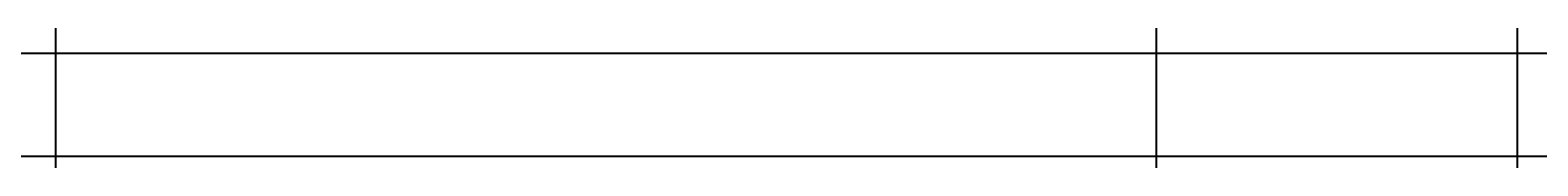
# Model space of a CAD drawing. Units: inches. Extents: x 35362 to 73946, y 43607 to 67532.
# Tile 79 of 134: x 50119 to 51337, y 47206 to 47304. Entities that reach past the tile are written whole.
import ezdxf

# ---------------------------------------------------------------- set-up
doc = ezdxf.new("R2010")
doc.units = ezdxf.units.IN
doc.header["$MEASUREMENT"] = 0
doc.layers.add('A-ANNO-DIMS', color=2, linetype='Continuous', lineweight=18)
doc.styles.get("Standard").update_dxf_attribs({"font": 'arial.ttf'})
doc.dimstyles.get("Standard").update_dxf_attribs({"dimtxt": 0.18, "dimasz": 0.18, "dimexe": 0.18, "dimexo": 0.0625, "dimgap": 0.09, "dimtad": 0, "dimtih": 1, "dimtoh": 1, "dimdec": 4, "dimzin": 0, "dimdsep": 46, "dimtxsty": 'Standard', "dimcen": 0.09, "dimadec": 0, "dimazin": 0, "dimtfac": 1, "dimtdec": 4, "dimtofl": 0, "dimtmove": 0, "dimatfit": 3, "dimfxl": 1, "dimtolj": 1, "dimtzin": 0, "dimarcsym": 0})

# ---------------------------------------------------------------- blocks, each defined once
blk = doc.blocks.new('*D11')
at = {"layer": 'A-ANNO-DIMS', "color": 0, "lineweight": -2, "transparency": 16777216}
for p, q in [((47978.7, 56028.8), (47978.7, 43606.7)), ((53109.8, 56028.8), (53109.8, 43606.7)), ((47978.8, 43606.9), (50543.9, 43606.9)), ((53109.6, 43606.9), (50544.6, 43606.9))]:
    blk.add_line(p, q, dxfattribs=at)
at = {"layer": 'A-ANNO-DIMS', "color": 0, "transparency": 16777216}
for points in [[(47978.8, 43606.9), (47978.8, 43606.8), (47978.7, 43606.9)], [(53109.6, 43606.9), (53109.6, 43606.8), (53109.8, 43606.9)]]:
    blk.add_solid(points, dxfattribs=at)
at = {"layer": 'Defpoints', "color": 0, "transparency": 16777216}
for p in [(47978.7, 56028.8), (53109.8, 56028.8), (53109.8, 43606.9)]:
    blk.add_point(p, dxfattribs=at)
at = {"layer": 'A-ANNO-DIMS', "color": 0, "transparency": 16777216, "insert": (50544.2, 43606.9), "char_height": 0.18, "attachment_point": 5}
blk.add_mtext('\\A1;5131', dxfattribs=at)
blk = doc.blocks.new('*D13')
at = {"layer": 'A-ANNO-DIMS', "color": 0, "lineweight": -2, "transparency": 16777216}
for p, q in [((48373.5, 51694), (48373.5, 43606.7)), ((51029, 51694), (51029, 43606.7)), ((48373.7, 43606.9), (49700.8, 43606.9)), ((51028.9, 43606.9), (49701.7, 43606.9))]:
    blk.add_line(p, q, dxfattribs=at)
at = {"layer": 'A-ANNO-DIMS', "color": 0, "transparency": 16777216}
for points in [[(48373.7, 43606.9), (48373.7, 43606.8), (48373.5, 43606.9)], [(51028.9, 43606.9), (51028.9, 43606.8), (51029, 43606.9)]]:
    blk.add_solid(points, dxfattribs=at)
at = {"layer": 'Defpoints', "color": 0, "transparency": 16777216}
for p in [(48373.5, 51694.1), (51029, 51694.1), (51029, 43606.9)]:
    blk.add_point(p, dxfattribs=at)
at = {"layer": 'A-ANNO-DIMS', "color": 0, "transparency": 16777216, "insert": (49701.3, 43606.9), "char_height": 0.18, "attachment_point": 5}
blk.add_mtext('\\A1;2655.6', dxfattribs=at)
blk = doc.blocks.new('*D17')
at = {"layer": 'A-ANNO-DIMS', "color": 0, "lineweight": -2, "transparency": 16777216}
for p, q in [((49923.3, 61293.2), (49923.3, 43606.7)), ((51913.9, 61293.2), (51913.9, 43606.7)), ((49923.5, 43606.9), (50918.2, 43606.9)), ((51913.8, 43606.9), (50919.1, 43606.9))]:
    blk.add_line(p, q, dxfattribs=at)
at = {"layer": 'A-ANNO-DIMS', "color": 0, "transparency": 16777216}
for points in [[(49923.5, 43606.9), (49923.5, 43606.8), (49923.3, 43606.9)], [(51913.8, 43606.9), (51913.8, 43606.8), (51913.9, 43606.9)]]:
    blk.add_solid(points, dxfattribs=at)
at = {"layer": 'Defpoints', "color": 0, "transparency": 16777216}
for p in [(49923.3, 61293.3), (51913.9, 61293.3), (51913.9, 43606.9)]:
    blk.add_point(p, dxfattribs=at)
at = {"layer": 'A-ANNO-DIMS', "color": 0, "transparency": 16777216, "insert": (50918.6, 43606.9), "char_height": 0.18, "attachment_point": 5}
blk.add_mtext('\\A1;1990.6', dxfattribs=at)
blk = doc.blocks.new('*D43')
at = {"layer": 'A-ANNO-DIMS', "color": 0, "lineweight": -2, "transparency": 16777216}
for p, q in [((62004.7, 47625.2), (35361.8, 47625.2)), ((35361.9, 47625), (35361.9, 47416.9)), ((35361.9, 47208.4), (35361.9, 47416.5)), ((62004.7, 47208.2), (35361.8, 47208.2))]:
    blk.add_line(p, q, dxfattribs=at)
at = {"layer": 'A-ANNO-DIMS', "color": 0, "transparency": 16777216}
for points in [[(35361.9, 47625), (35362, 47625), (35361.9, 47625.2)], [(35361.9, 47208.4), (35362, 47208.4), (35361.9, 47208.2)]]:
    blk.add_solid(points, dxfattribs=at)
at = {"layer": 'Defpoints', "color": 0, "transparency": 16777216}
for p in [(62004.7, 47625.2), (35361.9, 47208.2), (62004.7, 47208.2)]:
    blk.add_point(p, dxfattribs=at)
at = {"layer": 'A-ANNO-DIMS', "color": 0, "transparency": 16777216, "insert": (35361.9, 47416.7), "char_height": 0.18, "attachment_point": 5}
blk.add_mtext('\\A1;416.9', dxfattribs=at)
blk = doc.blocks.new('*D67')
at = {"layer": 'A-ANNO-DIMS', "color": 0, "lineweight": -2, "transparency": 16777216}
for p, q in [((56873.5, 53351.5), (35361.8, 53351.5)), ((35361.9, 53351.3), (35361.9, 49400.9)), ((35361.9, 45450.1), (35361.9, 49400.5)), ((53793.6, 45449.9), (35361.8, 45449.9))]:
    blk.add_line(p, q, dxfattribs=at)
at = {"layer": 'A-ANNO-DIMS', "color": 0, "transparency": 16777216}
for points in [[(35361.9, 53351.3), (35362, 53351.3), (35361.9, 53351.5)], [(35361.9, 45450.1), (35362, 45450.1), (35361.9, 45449.9)]]:
    blk.add_solid(points, dxfattribs=at)
at = {"layer": 'Defpoints', "color": 0, "transparency": 16777216}
for p in [(35361.9, 53351.5), (56873.6, 53351.5), (53793.6, 45449.9)]:
    blk.add_point(p, dxfattribs=at)
at = {"layer": 'A-ANNO-DIMS', "color": 0, "transparency": 16777216, "insert": (35361.9, 49400.7), "char_height": 0.18, "attachment_point": 5}
blk.add_mtext('\\A1;7901.6', dxfattribs=at)
blk = doc.blocks.new('*D90')
at = {"layer": 'A-ANNO-DIMS', "color": 0, "lineweight": -2, "transparency": 16777216}
for p, q in [((53707.7, 47291.3), (35361.8, 47291.3)), ((35361.9, 47291.1), (35361.9, 46710.3)), ((35361.9, 46129.1), (35361.9, 46709.9)), ((53793.6, 46128.9), (35361.8, 46128.9))]:
    blk.add_line(p, q, dxfattribs=at)
at = {"layer": 'A-ANNO-DIMS', "color": 0, "transparency": 16777216}
for points in [[(35361.9, 47291.1), (35362, 47291.1), (35361.9, 47291.3)], [(35361.9, 46129.1), (35362, 46129.1), (35361.9, 46128.9)]]:
    blk.add_solid(points, dxfattribs=at)
at = {"layer": 'Defpoints', "color": 0, "transparency": 16777216}
for p in [(53707.8, 47291.3), (35361.9, 46128.9), (53793.6, 46128.9)]:
    blk.add_point(p, dxfattribs=at)
at = {"layer": 'A-ANNO-DIMS', "color": 0, "transparency": 16777216, "insert": (35361.9, 46710.1), "char_height": 0.18, "attachment_point": 5}
blk.add_mtext('\\A1;1162.4', dxfattribs=at)
blk = doc.blocks.new('*D107')
at = {"layer": 'A-ANNO-DIMS', "color": 0, "lineweight": -2, "transparency": 16777216}
for p, q in [((50139.6, 59850), (50139.6, 43606.7)), ((51320.8, 59850), (51320.8, 43606.7)), ((50139.7, 43606.9), (50729.7, 43606.9)), ((51320.6, 43606.9), (50730.6, 43606.9))]:
    blk.add_line(p, q, dxfattribs=at)
at = {"layer": 'A-ANNO-DIMS', "color": 0, "transparency": 16777216}
for points in [[(50139.7, 43606.9), (50139.7, 43606.8), (50139.6, 43606.9)], [(51320.6, 43606.9), (51320.6, 43606.8), (51320.8, 43606.9)]]:
    blk.add_solid(points, dxfattribs=at)
at = {"layer": 'Defpoints', "color": 0, "transparency": 16777216}
for p in [(50139.6, 59850.1), (51320.8, 59850.1), (51320.8, 43606.9)]:
    blk.add_point(p, dxfattribs=at)
at = {"layer": 'A-ANNO-DIMS', "color": 0, "transparency": 16777216, "insert": (50730.2, 43606.9), "char_height": 0.18, "attachment_point": 5}
blk.add_mtext('\\A1;1181.3', dxfattribs=at)

msp = doc.modelspace()

# ---------------------------------------------------------------- dimensions: what is measured, and where the dimension line sits
at = {"layer": 'A-ANNO-DIMS'}
for base, p1, p2, override, picture, middle in [((51913.931, 43606.859), (49923.307, 61293.286), (51913.931, 61293.286), {"dimdec": 1, "dimlfac": 1, "dimrnd": 0, "dimzin": 0, "dimdsep": 46, "dimlunit": 2}, '*D17', (50918.619, 43606.859)), ((51320.8133, 43606.859), (50139.5627, 59850.0769), (51320.8133, 59850.0769), {"dimdec": 1, "dimlfac": 1, "dimrnd": 0, "dimzin": 0, "dimdsep": 46, "dimlunit": 2}, '*D107', (50730.188, 43606.859)), ((53109.76, 43606.859), (47978.665, 56028.836), (53109.76, 56028.836), {"dimdec": 0, "dimlfac": 1, "dimrnd": 0, "dimzin": 0, "dimdsep": 46, "dimlunit": 2}, '*D11', (50544.212, 43606.859)), ((51029.043, 43606.859), (48373.492, 51694.087), (51029.043, 51694.087), {"dimdec": 1, "dimlfac": 1, "dimrnd": 0, "dimzin": 0, "dimdsep": 46, "dimlunit": 2}, '*D13', (49701.267, 43606.859))]:
    dim = msp.add_linear_dim(base=base, p1=p1, p2=p2, dimstyle='Standard', override=override, dxfattribs=at)
    dim.commit()
    dim.dimension.update_dxf_attribs({"geometry": picture, "text_midpoint": middle})
for base, p1, p2, picture, middle in [((35361.949, 53351.529), (53793.638, 45449.894), (56873.602, 53351.529), '*D67', (35361.949, 49400.712)), ((35361.949, 47208.25), (62004.728, 47625.181), (62004.728, 47208.25), '*D43', (35361.949, 47416.715)), ((35361.949, 46128.878), (53707.781, 47291.285), (53793.638, 46128.878), '*D90', (35361.949, 46710.081))]:
    dim = msp.add_linear_dim(base=base, p1=p1, p2=p2, angle=90, dimstyle='Standard', override={"dimdec": 1, "dimlfac": 1, "dimrnd": 0, "dimzin": 0, "dimdsep": 46, "dimlunit": 2}, dxfattribs=at)
    dim.commit()
    dim.dimension.update_dxf_attribs({"geometry": picture, "text_midpoint": middle})

doc.saveas('drawing.dxf')
